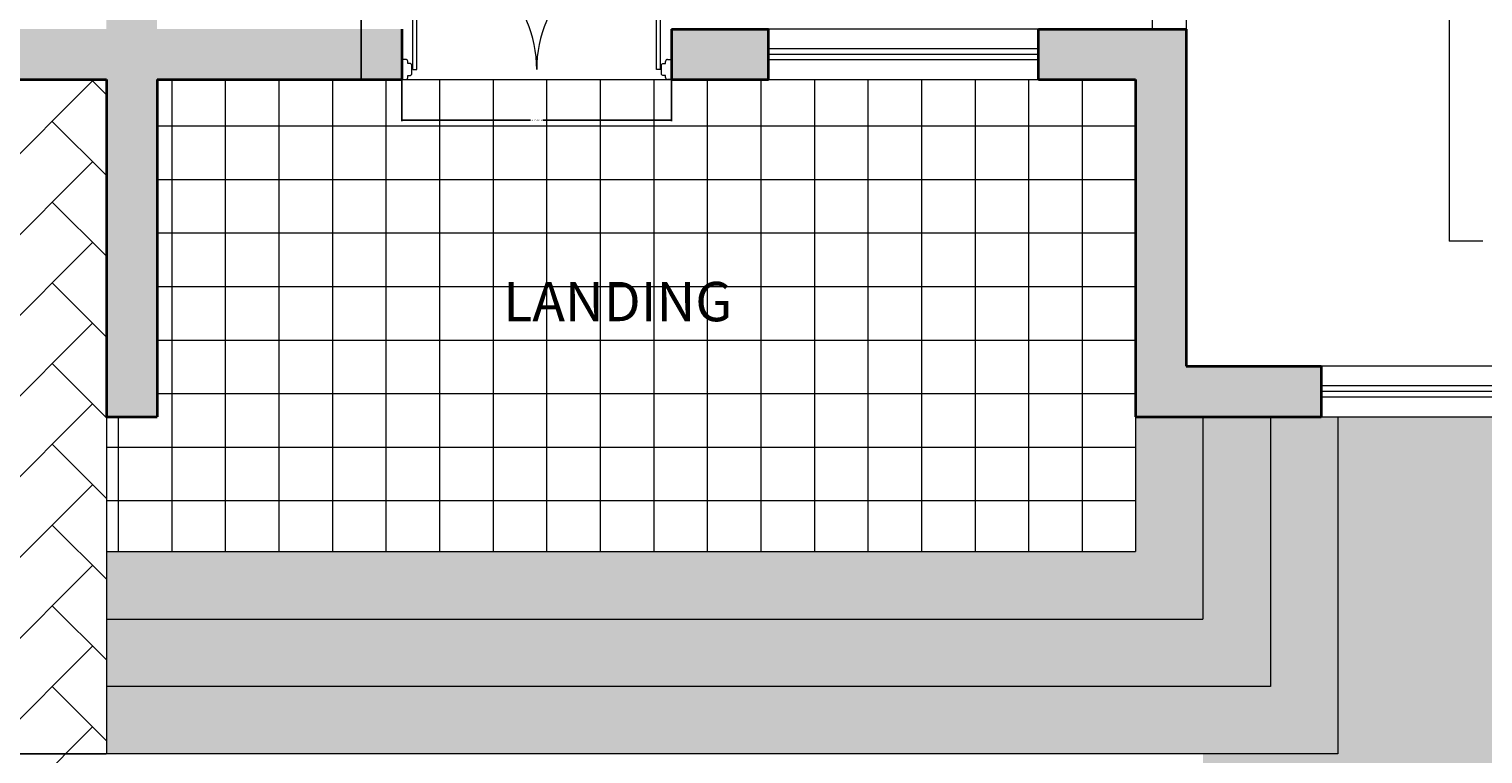
# Model space of a CAD drawing. Units: inches. Extents: x 84 to 1044, y -280 to 906.
# Tile 21 of 105: x 441 to 700, y 31 to 160. Entities that reach past the tile are written whole.
import ezdxf

# ---------------------------------------------------------------- set-up
doc = ezdxf.new("R2010")
doc.units = ezdxf.units.IN
doc.linetypes.add('ACAD_ISO02W100', pattern=[15, 12, -3])
for name, color, linetype, lineweight in [('00 FURNITURE', 15, 'Continuous', 15), ('A-ANNO-DIMS', 2, 'Continuous', 18), ('A-AREA-IDEN', 7, 'Continuous', 13), ('A-DOOR', 4, 'Continuous', 18), ('A-FURN', 8, 'Continuous', 15), ('A-STAIRCASE', 144, 'Continuous', 18), ('A-WALL-OVHD', 8, 'ACAD_ISO02W100', 13), ('WALL', 250, 'Continuous', 35), ('WINDOW', 160, 'Continuous', 13)]:
    doc.layers.add(name, color=color, linetype=linetype, lineweight=lineweight)
for name, color, linetype, lineweight, true_color in [('A-FLOR-PATT', 251, 'Continuous', 9, 0x705861), ('A-FLOR-STRS-PATT', 35, 'Continuous', 9, 0x947764), ('A-WALL-PATT', 251, 'Continuous', 9, 0x636466), ('L-PLNT-PATT', 9, 'Continuous', 9, 0xafd9aa), ('L-PRKG-PATT', 35, 'Continuous', 9, 0x947764)]:
    doc.layers.add(name, color=color, linetype=linetype, lineweight=lineweight, true_color=true_color)
doc.styles.add('1-100DIM', font='txt', dxfattribs={"height": 0.3})
doc.styles.get("Standard").update_dxf_attribs({"font": 'arial.ttf'})
doc.dimstyles.get("Standard").update_dxf_attribs({"dimtxt": 0.18, "dimasz": 0.18, "dimexe": 0.18, "dimexo": 0.0625, "dimgap": 0.09, "dimtad": 0, "dimtih": 1, "dimtoh": 1, "dimdec": 4, "dimzin": 0, "dimdsep": 46, "dimtxsty": 'Standard', "dimcen": 0.09, "dimadec": 0, "dimazin": 0, "dimtfac": 1, "dimtdec": 4, "dimtofl": 0, "dimtmove": 0, "dimatfit": 3, "dimfxl": 1, "dimtolj": 1, "dimtzin": 0, "dimarcsym": 0})

# ---------------------------------------------------------------- blocks, each defined once
blk = doc.blocks.new('PUJA')
at = {"layer": '00 FURNITURE'}
for p, q in [((-1940.35, -16093.35), (-1958.14, -16093.35)), ((-1941.8, -16091.75), (-1938.89, -16091.75)), ((-1941.8, -16092.33), (-1941.8, -16091.75)), ((-1941.22, -16092.62), (-1941.51, -16092.62)), ((-1940.35, -16093.35), (-1940.35, -16093.93)), ((-1939.18, -16092.62), (-1939.47, -16092.62)), ((-1938.89, -16091.75), (-1938.89, -16092.33)), ((-1940.35, -16093.93), (-1958.13, -16093.93)), ((-1940.35, -16128.93), (-1958.14, -16128.93)), ((-1940.35, -16128.35), (-1958.13, -16128.35)), ((-1940.35, -16128.93), (-1940.35, -16128.35)), ((-1941.8, -16129.96), (-1941.8, -16130.54)), ((-1941.8, -16130.54), (-1938.89, -16130.54)), ((-1941.22, -16129.66), (-1941.51, -16129.66)), ((-1939.18, -16129.66), (-1939.47, -16129.66)), ((-1938.89, -16130.54), (-1938.89, -16129.96))]:
    blk.add_line(p, q, dxfattribs=at)
for points in [[(-1939.47, -16092.62), (-1939.47, -16092.91, -0.414214), (-1939.76, -16093.21), (-1940.93, -16093.21, -0.414214), (-1941.22, -16092.91), (-1941.22, -16092.62)], [(-1939.47, -16129.66), (-1939.47, -16129.37, 0.414214), (-1939.76, -16129.08), (-1940.93, -16129.08, 0.414214), (-1941.22, -16129.37), (-1941.22, -16129.66)]]:
    blk.add_lwpolyline(points, format="xyb", dxfattribs=at)
for centre, radius, start, end in [((-1940.35, -16093.35), 17.79, 180, 270), ((-1941.51, -16092.33), 0.292, 180, 270), ((-1939.18, -16092.33), 0.292, 270, 0), ((-1940.35, -16128.93), 17.79, 90, 180), ((-1941.51, -16129.96), 0.292, 90, 180), ((-1939.18, -16129.96), 0.292, 0, 90)]:
    blk.add_arc(centre, radius, start, end, dxfattribs=at)
blk = doc.blocks.new('WIN-72IN')
for p, q in [((72, 9), (0, 9)), ((72, 5.5), (0, 5.5)), ((72, 4.5), (0, 4.5)), ((72, 3.5), (0, 3.5)), ((0, 0), (72, 0))]:
    blk.add_line(p, q)
blk = doc.blocks.new('*D42')
at = {"layer": 'A-ANNO-DIMS', "color": 0, "lineweight": -2, "transparency": 16777216}
for p, q in [((507.57, 151.06), (507.57, 143.74)), ((555.57, 151.06), (555.57, 143.74)), ((507.75, 143.92), (530.49, 143.92)), ((555.39, 143.92), (532.66, 143.92))]:
    blk.add_line(p, q, dxfattribs=at)
at = {"layer": 'A-ANNO-DIMS', "color": 0, "transparency": 16777216}
for points in [[(507.75, 143.95), (507.75, 143.89), (507.57, 143.92)], [(555.39, 143.95), (555.39, 143.89), (555.57, 143.92)]]:
    blk.add_solid(points, dxfattribs=at)
at = {"layer": 'Defpoints', "color": 0, "transparency": 16777216}
for p in [(507.57, 151.12), (555.57, 151.12), (555.57, 143.92)]:
    blk.add_point(p, dxfattribs=at)
at = {"layer": 'A-ANNO-DIMS', "color": 0, "transparency": 16777216, "insert": (531.57, 143.92), "char_height": 0.18, "attachment_point": 5}
blk.add_mtext('\\A1;ENTRY DOOR 48', dxfattribs=at)
blk = doc.blocks.new('*D43')
at = {"layer": 'A-ANNO-DIMS', "color": 0, "lineweight": -2, "transparency": 16777216}
for p, q in [((507.51, 174.94), (500.19, 174.94)), ((500.37, 174.76), (500.37, 163.21)), ((500.37, 151.3), (500.37, 162.85)), ((507.51, 151.12), (500.19, 151.12))]:
    blk.add_line(p, q, dxfattribs=at)
at = {"layer": 'A-ANNO-DIMS', "color": 0, "transparency": 16777216}
for points in [[(500.34, 174.76), (500.4, 174.76), (500.37, 174.94)], [(500.34, 151.3), (500.4, 151.3), (500.37, 151.12)]]:
    blk.add_solid(points, dxfattribs=at)
at = {"layer": 'Defpoints', "color": 0, "transparency": 16777216}
for p in [(507.57, 174.94), (500.37, 151.12), (507.57, 151.12)]:
    blk.add_point(p, dxfattribs=at)
at = {"layer": 'A-ANNO-DIMS', "color": 0, "transparency": 16777216, "insert": (500.37, 163.03), "char_height": 0.18, "attachment_point": 5}
blk.add_mtext('\\A1;24', dxfattribs=at)
blk = doc.blocks.new('*D80')
at = {"layer": 'A-ANNO-DIMS', "color": 0, "lineweight": -2, "transparency": 16777216}
for p, q in [((455.01, 151.12), (405.29, 151.12)), ((405.47, 150.94), (405.47, 91.3)), ((405.47, 31.3), (405.47, 90.94)), ((455.01, 31.12), (405.29, 31.12))]:
    blk.add_line(p, q, dxfattribs=at)
at = {"layer": 'A-ANNO-DIMS', "color": 0, "transparency": 16777216}
for points in [[(405.44, 150.94), (405.5, 150.94), (405.47, 151.12)], [(405.44, 31.3), (405.5, 31.3), (405.47, 31.12)]]:
    blk.add_solid(points, dxfattribs=at)
at = {"layer": 'Defpoints', "color": 0, "transparency": 16777216}
for p in [(405.47, 151.12), (455.07, 151.12), (455.07, 31.12)]:
    blk.add_point(p, dxfattribs=at)
at = {"layer": 'A-ANNO-DIMS', "color": 0, "transparency": 16777216, "insert": (405.47, 91.12), "char_height": 0.18, "attachment_point": 5}
blk.add_mtext('\\A1;120', dxfattribs=at)

msp = doc.modelspace()

# ---------------------------------------------------------------- hatches: boundary and pattern name
at = {"layer": 'A-FLOR-PATT', "transparency": 33554597}
h = msp.add_hatch(dxfattribs=at)
h.set_pattern_fill('ANSI37', color=256, scale=3, angle=45)
h.paths.add_polyline_path([(638.074, 151.12), (620.824, 151.12), (572.824, 151.12), (555.574, 151.12), (507.574, 151.12), (464.074, 151.12), (464.074, 91.12), (455.074, 91.12), (455.074, 67.12), (638.074, 67.12), (638.074, 91.12)])
at = {"layer": 'A-FLOR-STRS-PATT', "transparency": 33554567}
h = msp.add_hatch(color=256, dxfattribs=at)
h.dxf.hatch_style = 1
h.paths.add_polyline_path([(650.074, 91.12), (638.074, 91.12), (638.074, 67.12), (455.074, 67.12), (455.074, 55.12), (650.074, 55.12)], flags=17)
h.paths.add_polyline_path([(662.074, 91.12), (650.074, 91.12), (650.074, 55.12), (455.074, 55.12), (455.074, 43.12), (662.074, 43.12)])
h.paths.add_polyline_path([(674.074, 91.12), (671.074, 91.12), (662.074, 91.12), (662.074, 43.12), (455.074, 43.12), (455.074, 31.12), (674.074, 31.12)])
h.paths.add_polyline_path([(227.179, 151.12), (203.179, 151.12), (143.179, 151.12), (143.179, 139.12), (227.179, 139.12)])
h.paths.add_polyline_path([(227.179, 139.12), (143.179, 139.12), (143.179, 127.12), (227.179, 127.12)])
h.paths.add_polyline_path([(203.179, 271.12), (143.179, 271.12), (143.179, 259.12), (203.179, 259.12)])
h.paths.add_polyline_path([(203.179, 259.12), (143.179, 259.12), (143.179, 247.12), (203.179, 247.12)])
h.paths.add_polyline_path([(203.179, 769.12), (143.179, 769.12), (143.179, 757.12), (203.179, 757.12)])
h.paths.add_polyline_path([(203.179, 757.12), (143.179, 757.12), (143.179, 745.12), (203.179, 745.12)])
h.paths.add_polyline_path([(434.074, 847.12), (422.074, 847.12), (422.074, 769.12), (434.074, 769.12)])
h.paths.add_polyline_path([(422.074, 847.12), (410.074, 847.12), (410.074, 769.12), (422.074, 769.12)])
at = {"layer": 'A-WALL-PATT', "transparency": 33554597}
h = msp.add_hatch(color=256, dxfattribs=at)
h.dxf.hatch_style = 1
h.paths.add_polyline_path([(671.074, 100.12), (647.074, 100.12), (647.074, 160.12), (641.074, 160.12), (620.824, 160.12), (620.824, 151.12), (638.074, 151.12), (638.074, 91.12), (671.074, 91.12)])
h.paths.add_polyline_path([(791.074, 100.12), (743.074, 100.12), (743.074, 91.12), (791.074, 91.12)])
h.paths.add_polyline_path([(896.074, 346.12), (887.074, 346.12), (887.074, 334.12), (870.955, 334.12), (833.074, 334.12), (804.574, 334.12), (804.574, 328.12), (887.074, 328.12), (887.074, 100.12), (863.074, 100.12), (863.074, 91.12), (896.074, 91.12)])
h.paths.add_polyline_path([(507.574, 154.729), (507.574, 160.12), (464.074, 160.12), (464.074, 247.12), (641.074, 247.12), (641.074, 208.12), (647.074, 208.12), (647.074, 328.12), (659.074, 328.12), (659.074, 334.12), (617.074, 334.12), (617.074, 328.12), (641.074, 328.12), (641.074, 256.12), (545.074, 256.12), (545.074, 328.12), (569.074, 328.12), (569.074, 334.12), (518.074, 334.12), (518.074, 325.12), (536.074, 325.12), (536.074, 256.12), (464.074, 256.12), (464.074, 325.12), (482.074, 325.12), (482.074, 334.12), (455.074, 334.12), (455.074, 160.12), (413.127, 160.12), (413.127, 151.12), (455.074, 151.12), (455.074, 91.12), (464.074, 91.12), (464.074, 151.12), (507.574, 151.12)])
h.paths.add_polyline_path([(572.824, 160.12), (555.574, 160.12), (555.574, 151.12), (572.824, 151.12)], flags=17)
h.paths.add_polyline_path([(341.127, 160.12), (299.179, 160.12), (299.179, 211.12), (294.179, 211.12), (290.179, 211.12), (290.179, 151.12), (341.127, 151.12)])
h.paths.add_polyline_path([(299.179, 256.12), (212.179, 256.12), (212.179, 274.12), (203.179, 274.12), (203.179, 247.12), (299.179, 247.12)])
h.paths.add_polyline_path([(212.179, 514.12), (398.074, 514.12), (398.074, 519.12), (398.074, 520.12), (212.179, 520.12), (212.179, 574.12), (203.179, 574.12), (203.179, 310.12), (212.179, 310.12), (212.179, 328.12), (290.179, 328.12), (290.179, 292.12), (299.179, 292.12), (299.179, 328.12), (332.179, 328.12), (332.179, 334.12), (212.179, 334.12)])
h.paths.add_polyline_path([(287.127, 709.12), (203.179, 709.12), (203.179, 646.12), (212.179, 646.12), (212.179, 700.12), (287.127, 700.12)])
h.paths.add_polyline_path([(470.074, 709.12), (359.127, 709.12), (359.127, 700.12), (434.074, 700.12), (434.074, 574.12), (440.074, 574.12), (440.074, 622.12), (464.074, 622.12), (464.074, 628.12), (440.074, 628.12), (440.074, 700.12), (470.074, 700.12)])
h.paths.add_polyline_path([(572.074, 709.12), (506.074, 709.12), (506.074, 700.12), (536.074, 700.12), (536.074, 628.12), (494.074, 628.12), (494.074, 622.12), (536.074, 622.12), (536.074, 520.12), (440.074, 520.12), (440.074, 544.12), (434.074, 544.12), (434.074, 514.12), (644.074, 514.12), (644.074, 519.12), (644.074, 544.12), (638.074, 544.12), (638.074, 520.12), (542.074, 520.12), (542.074, 622.12), (584.074, 622.12), (584.074, 628.12), (542.074, 628.12), (542.074, 700.12), (572.074, 700.12)])
h.paths.add_polyline_path([(698.074, 709.12), (608.074, 709.12), (608.074, 700.12), (638.074, 700.12), (638.074, 628.12), (614.074, 628.12), (614.074, 622.12), (638.074, 622.12), (638.074, 574.12), (644.074, 574.12), (644.074, 700.12), (698.074, 700.12)])
h.paths.add_polyline_path([(833.074, 709.12), (770.074, 709.12), (770.074, 700.12), (824.074, 700.12), (824.074, 646.12), (833.074, 646.12)])
h.paths.add_polyline_path([(833.074, 574.12), (824.074, 574.12), (824.074, 520.12), (791.244, 520.12), (712.904, 520.12), (680.074, 520.12), (680.074, 514.12), (695.074, 514.12), (695.074, 491.62), (704.074, 491.62), (704.074, 511.12), (833.074, 511.12)])
h.paths.add_polyline_path([(704.074, 419.62), (695.074, 419.62), (695.074, 370.12), (704.074, 370.12)])
h.paths.add_polyline_path([(896.074, 400.12), (833.074, 400.12), (833.074, 364.12), (839.074, 364.12), (839.074, 394.12), (887.074, 394.12), (887.074, 382.12), (896.074, 382.12)])
h.paths.add_polyline_path([(732.574, 334.12), (695.074, 334.12), (695.074, 328.12), (732.574, 328.12)])
at = {"layer": 'L-PLNT-PATT', "transparency": 33554597}
h = msp.add_hatch(color=256, dxfattribs=at)
h.dxf.hatch_style = 1
h.paths.add_polyline_path([(791.074, 31.12), (791.074, 91.12), (743.074, 91.12), (674.074, 91.12), (674.074, 31.12), (650.074, 31.12), (650.074, -112.88), (983.074, -112.88), (983.074, -64.88), (791.074, -64.88)])
at = {"layer": 'L-PRKG-PATT', "transparency": 33554567}
h = msp.add_hatch(dxfattribs=at)
h.set_pattern_fill('AR-HBONE', color=256, scale=0.1)
h.paths.add_polyline_path([(455.074, 31.12), (455.074, 91.12), (455.074, 151.12), (413.127, 151.12), (341.127, 151.12), (290.179, 151.12), (227.179, 151.12), (227.179, 127.12), (143.179, 127.12), (143.179, -112.88), (143.179, -117.88), (455.074, -117.88)])

# ---------------------------------------------------------------- linework, layer by layer
at = {"layer": 'A-DOOR'}
msp.add_line((507.574, 151.12), (555.574, 151.12), dxfattribs=at)
at = {"layer": 'A-FURN'}
for p in [(693.863, 307.895), (699.863, 122.358)]:
    msp.add_line(p, (693.863, 122.358), dxfattribs=at)
at = {"layer": 'A-STAIRCASE'}
for p, q in [((455.074, 91.12), (455.074, 31.12)), ((638.074, 91.12), (638.074, 67.12)), ((650.074, 91.12), (650.074, 55.12)), ((455.074, 67.12), (638.074, 67.12)), ((455.074, 55.12), (650.074, 55.12))]:
    msp.add_line(p, q, dxfattribs=at)
for points in [[(662.074, 91.12), (662.074, 43.12), (455.074, 43.12)], [(674.074, 91.12), (674.074, 31.12), (455.074, 31.12)]]:
    msp.add_lwpolyline(points, dxfattribs=at)
at = {"layer": 'A-WALL-OVHD'}
msp.add_lwpolyline([(641.074, 208.12), (647.074, 208.12), (647.074, 160.12), (641.074, 160.12)], close=True, dxfattribs=at)
at = {"layer": 'WALL'}
for p, q in [((507.574, 160.12), (507.574, 151.12)), ((555.574, 160.12), (555.574, 151.12)), ((555.574, 160.12), (572.824, 160.12)), ((572.824, 151.12), (572.824, 160.12)), ((620.824, 151.12), (620.824, 160.12)), ((620.824, 160.12), (647.074, 160.12)), ((647.074, 160.12), (647.074, 100.12)), ((413.127, 151.12), (455.074, 151.12)), ((455.074, 151.12), (455.074, 91.12)), ((464.074, 151.12), (507.574, 151.12)), ((464.074, 151.12), (464.074, 91.12)), ((555.574, 151.12), (572.824, 151.12)), ((620.824, 151.12), (638.074, 151.12)), ((638.074, 151.12), (638.074, 91.12)), ((647.074, 100.12), (671.074, 100.12)), ((671.074, 100.12), (671.074, 91.12)), ((455.074, 91.12), (464.074, 91.12)), ((638.074, 91.12), (671.074, 91.12))]:
    msp.add_line(p, q, dxfattribs=at)
at = {"layer": 'WINDOW'}
for p, q in [((620.824, 160.12), (572.824, 160.12)), ((620.824, 156.62), (572.824, 156.62)), ((620.824, 155.62), (572.824, 155.62)), ((620.824, 154.62), (572.824, 154.62)), ((572.824, 151.12), (620.824, 151.12))]:
    msp.add_line(p, q, dxfattribs=at)

# ---------------------------------------------------------------- block references
at = {"layer": 'A-DOOR', "xscale": 1.237379162154587, "yscale": 1.237379162154587, "zscale": 1.237379162154587, "rotation": 270.0000000034012}
msp.add_blockref('PUJA', (20467.167, -2248.02), dxfattribs=at)
at = {"layer": 'WINDOW'}
msp.add_blockref('WIN-72IN', (671.07, 91.12), dxfattribs=at)

# ---------------------------------------------------------------- texts
at = {"layer": 'A-AREA-IDEN', "insert": (521.342, 115.125), "char_height": 7, "attachment_point": 1, "style": '1-100DIM'}
msp.add_mtext_dynamic_manual_height_columns('{\\f@Malgun Gothic|b0|i0|c0|p34;  LANDING}', width=54.16989, gutter_width=15.851, heights=[0], dxfattribs=at)

# ---------------------------------------------------------------- dimensions: what is measured, and where the dimension line sits
at = {"layer": 'A-ANNO-DIMS'}
for base, p1, p2, angle, picture, middle in [((500.374, 151.12), (507.574, 174.94), (507.574, 151.12), 270, '*D43', (500.374, 163.03)), ((405.474, 151.12), (455.074, 31.12), (455.074, 151.12), 90, '*D80', (405.474, 91.12))]:
    dim = msp.add_linear_dim(base=base, p1=p1, p2=p2, angle=angle, dimstyle='Standard', override={"dimdec": 0, "dimlfac": 1, "dimrnd": 0, "dimzin": 0, "dimdsep": 46, "dimlunit": 2}, dxfattribs=at)
    dim.commit()
    dim.dimension.update_dxf_attribs({"geometry": picture, "text_midpoint": middle})
dim = msp.add_linear_dim(base=(555.574, 143.92), p1=(507.574, 151.12), p2=(555.574, 151.12), angle=0, text='ENTRY DOOR <>', dimstyle='Standard', override={"dimdec": 0, "dimlfac": 1, "dimrnd": 0, "dimzin": 0, "dimdsep": 46, "dimlunit": 2}, dxfattribs=at)
dim.commit()
dim.dimension.update_dxf_attribs({"geometry": '*D42', "text_midpoint": (531.574, 143.92)})

doc.saveas('drawing.dxf')
